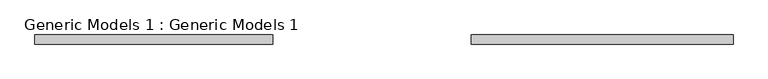
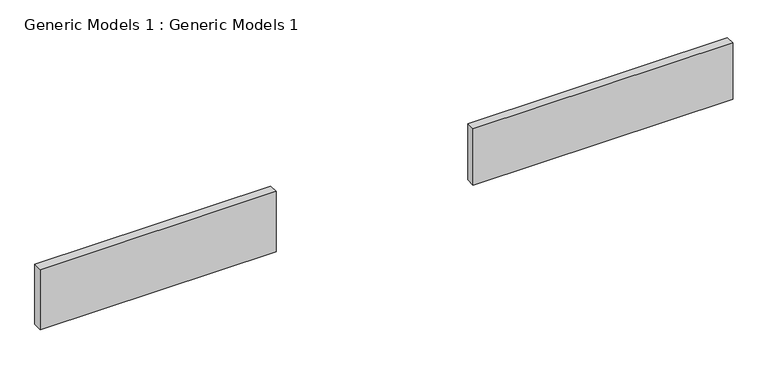
"""IFC4 building model written with IfcOpenShell, lengths in millimetres: proxy geometry, Generic Models 1 : Generic Models 1."""

from ifc_helpers import new_model, si_unit, frame, origin, place, context, project, spatial, polyline, outline, extrude, source, transform, mapped, element, save


def generic_models_1_generic_models_1_75855b24(model_context):
    return source(origin(), model_context, "Body", "SweptSolid", [
        extrude(outline(polyline([(5430.4022658, -8287.3061589), (1067.7345986, -8287.3061589), (1067.7345986, -8134.9061589), (5430.4022658, -8134.9061589), (5430.4022658, -8287.3061589)])), frame((0.0, 0.0, 227.3543205), z_axis=(0.0, 0.0, 1.0), x_axis=(1.0, 0.0, 0.0)), (0.0, 0.0, 1.0), 1000.9548608),
        extrude(outline(polyline([(-2248.5199368, -8287.3061589), (-6210.9199368, -8287.3061589), (-6210.9199368, -8134.9061589), (-2248.5199368, -8134.9061589), (-2248.5199368, -8287.3061589)])), frame((0.0, 0.0, 207.7335756), z_axis=(0.0, 0.0, 1.0), x_axis=(1.0, 0.0, 0.0)), (0.0, 0.0, 1.0), 1066.8),
    ])


if __name__ == "__main__":
    model = new_model("IFC4")
    model_context = context("Model", 3, world=origin())
    ifc_project = project(units=[si_unit("LENGTHUNIT", "METRE", prefix="MILLI")], contexts=[model_context])
    site = spatial("IfcSite", under=ifc_project)
    building = spatial("IfcBuilding", under=site)
    placement = place(None, origin())
    generic_models_1_generic_models_1_shape = generic_models_1_generic_models_1_75855b24(model_context)
    element("IfcBuildingElementProxy", 1, Name="Generic Models 1 : Generic Models 1", ObjectType="Generic Models 1 : Generic Models 1", at=placement, inside=building, context=model_context, shape_type="MappedRepresentation", body=[
        mapped(generic_models_1_generic_models_1_shape, transform((0.0, 0.0, 0.0), x_axis=(1.0, 0.0, 0.0), y_axis=(0.0, 1.0, 0.0), z_axis=(0.0, 0.0, 1.0))),
    ])
    save(model, "model.ifc")

# Revit data of these elements
# Element 1 (IfcBuildingElementProxy, "Generic Models 1 : Generic Models 1")
#   Materials on its faces: "Parking Stripe"
# Materials
#   "Parking Stripe": class "Paint", colour RGB 250 250 91, transparency 0, Cost = 0
